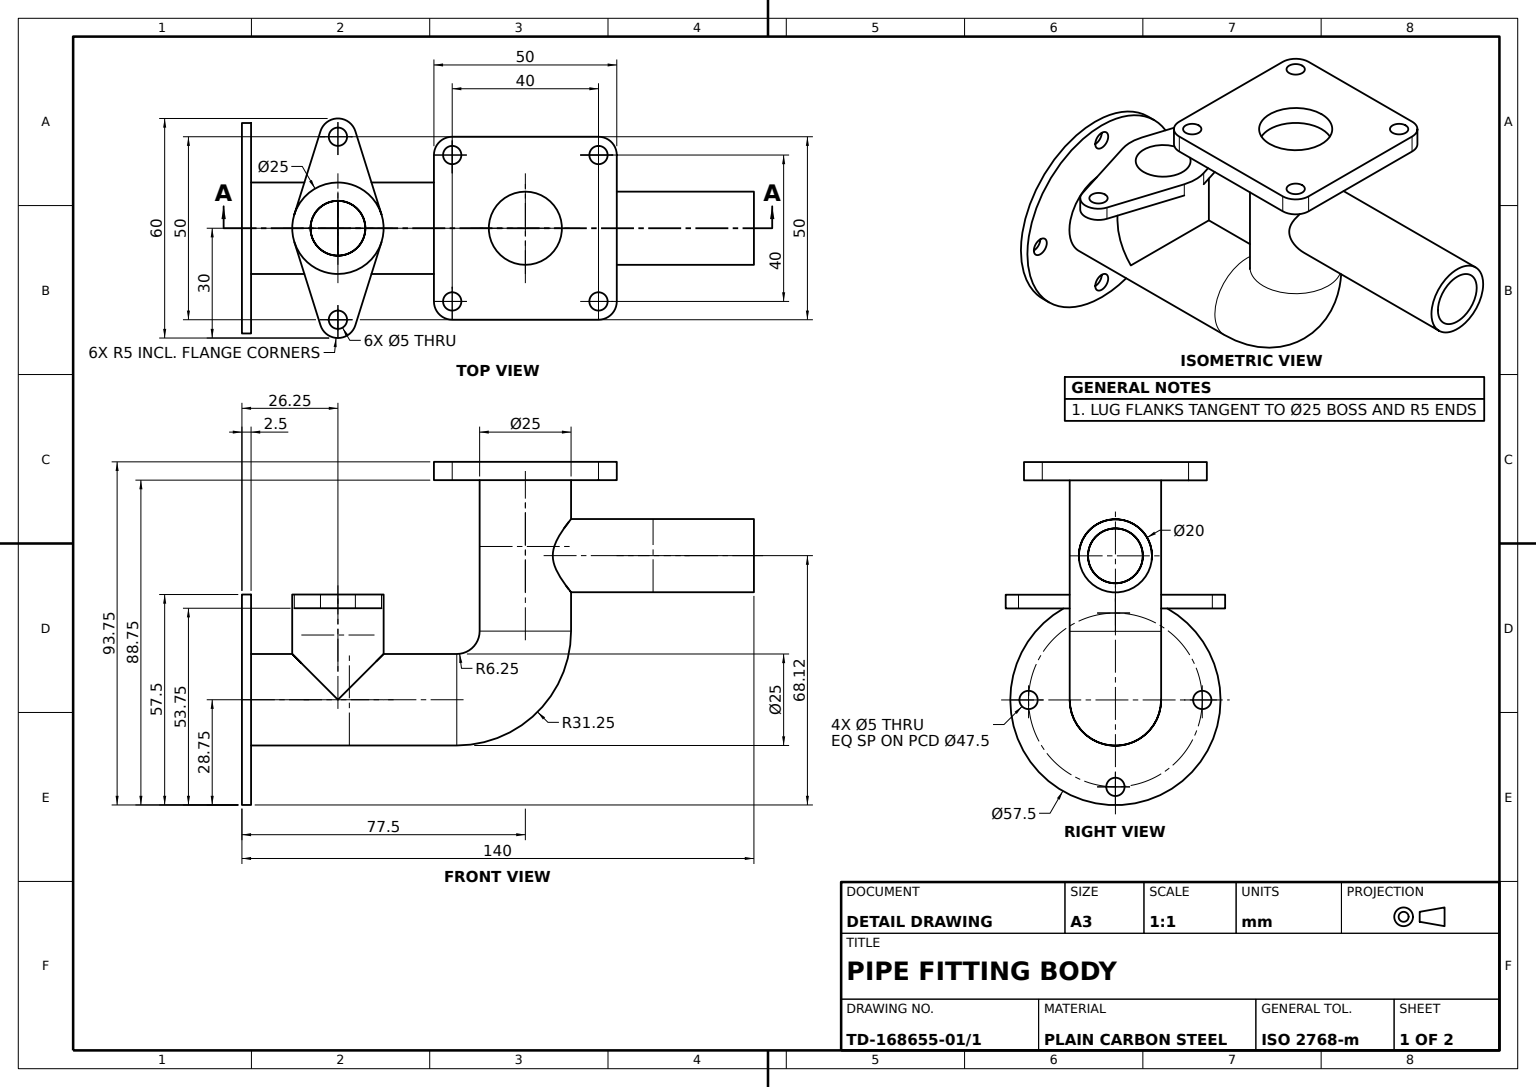
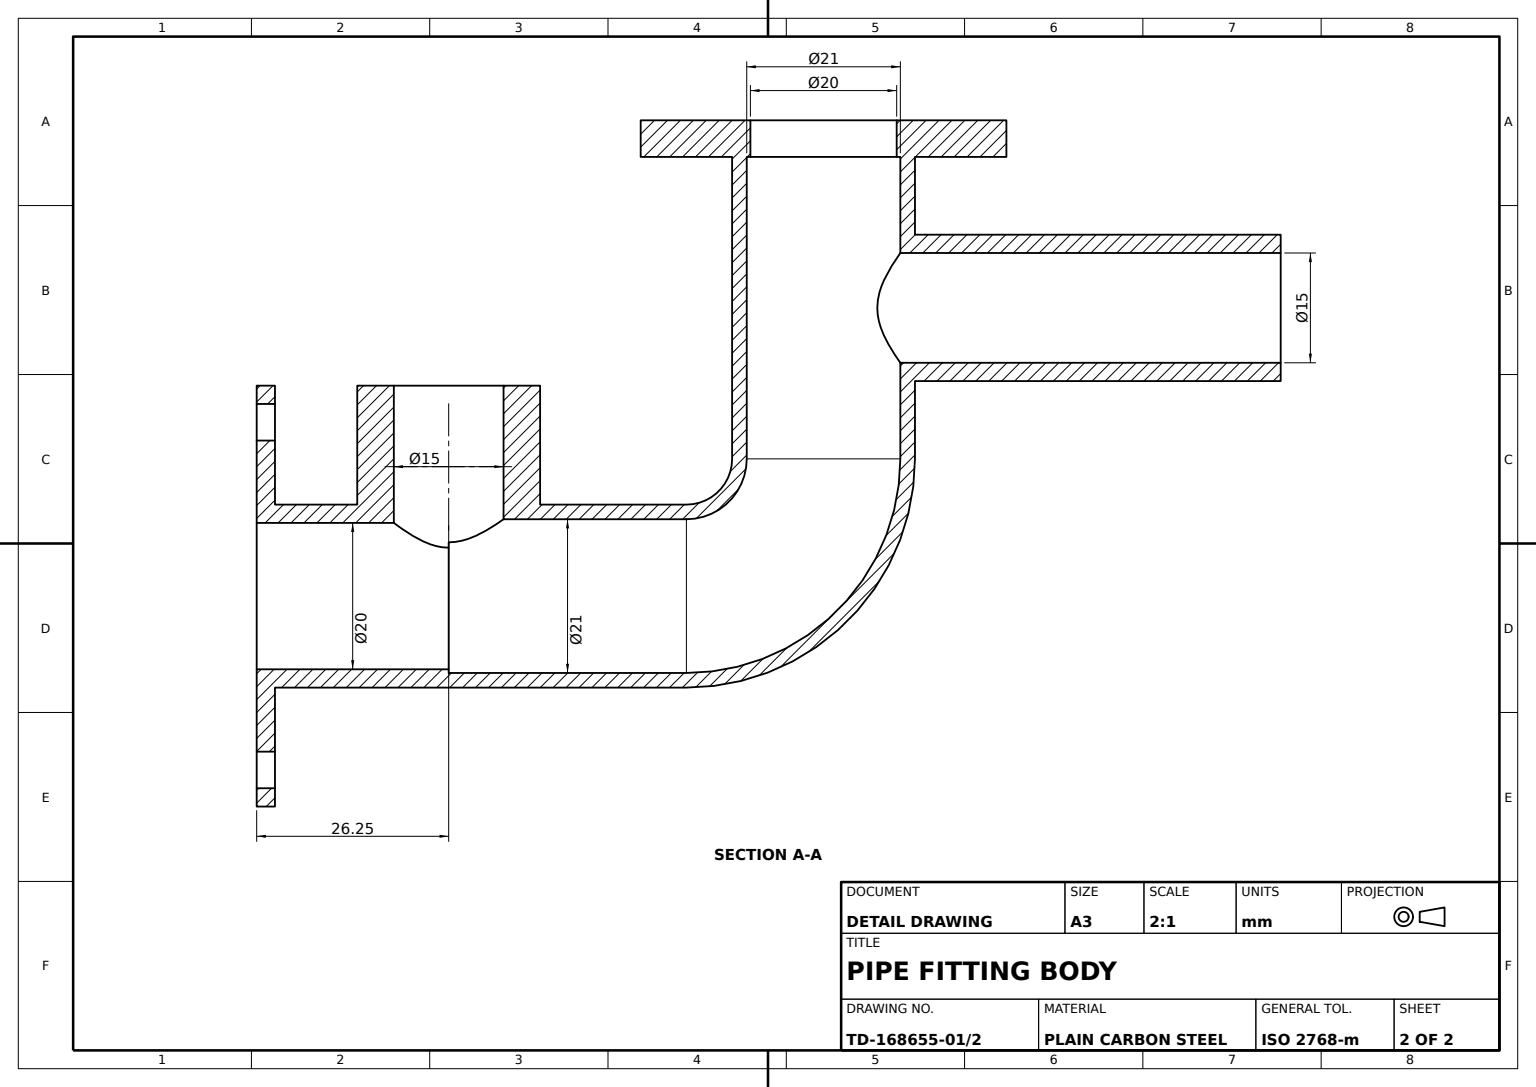
from build123d import *

# Parameters (mm, degrees)
ROUND_FLANGE_SKETCH_R         = 28.75
ROUND_FLANGE_57_5_DEPTH       = 2.5
INLET_PIPE_SKETCH_R           = 10
INLET_PIPE_20_DEPTH           = 23.75
FLANGE_A_NECK_REACH           = 71.44
FLANGE_A_NECK_END_RADIUS      = 10
FLANGE_A_NECK_SKETCH_R        = 10
FLANGE_A_HUB_SKETCH_R         = 12.5
FLANGE_A_HUB_25_DEPTH         = 3.75
FLANGE_A_LUG_1_SKETCH_R       = 5
FLANGE_A_LUG_1_DEPTH          = 3.75
FLANGE_A_LUG_2_SKETCH_R       = 5
FLANGE_A_LUG_2_DEPTH          = 3.75
FLANGE_A_WEB_25X10_DEPTH      = 3.75
FLANGE_A_TRIM_SKETCH_W        = 46.981578054
FLANGE_A_TRIM_SKETCH_H        = 84.080147296
FLANGE_A_TRIM_CUT_DEPTH       = 80
OUTLET_PIPE_SKETCH_R          = 12.5
OUTLET_PIPE_25_DEPTH          = 23.75
FLANGE_B_HUB_25_REACH         = 71.44
FLANGE_B_HUB_25_END_RADIUS    = 12.5
FLANGE_B_HUB_SKETCH_R         = 12.5
FLANGE_B_LUG_1_SKETCH_R       = 5
FLANGE_B_LUG_1_DEPTH          = 3.75
FLANGE_B_LUG_2_SKETCH_R       = 5
FLANGE_B_LUG_2_DEPTH          = 3.75
FLANGE_B_WEB_1_25X10_DEPTH    = 3.75
FLANGE_B_WEB_2_10X25_DEPTH    = 3.75
FLANGE_B_LUG_1_HOLE_SKETCH_R  = 2.5
FLANGE_B_LUG_1_HOLE_5_DEPTH   = 16.75
FLANGE_B_LUG_2_HOLE_SKETCH_R  = 2.5
FLANGE_B_LUG_2_HOLE_5_DEPTH   = 16.75
ELBOW_PIPE_SWEEP_PROFILE_R    = 12.5
ELBOW_PIPE_SWEEP_PROFILE_R_2  = 10.5
SQUARE_FLANGE_50X50_DEPTH     = 5
ROUND_FLANGE_BORE_SKETCH_R    = 10
ROUND_FLANGE_BORE_DEPTH       = 58
FLANGE_B_BORE_SKETCH_R        = 7.5
FLANGE_B_BORE_15_DEPTH        = 26
SQUARE_FLANGE_BORE_SKETCH_R   = 10
SQUARE_FLANGE_BORE_20_DEPTH   = 26
SQUARE_FLANGE_HOLE_1_SKETCH_R = 2.5
SQUARE_FLANGE_HOLE_1_5_DEPTH  = 26
SQUARE_FLANGE_HOLE_2_SKETCH_R = 2.5
SQUARE_FLANGE_HOLE_2_5_DEPTH  = 26
SQUARE_FLANGE_HOLE_3_SKETCH_R = 2.5
SQUARE_FLANGE_HOLE_3_5_DEPTH  = 26
SQUARE_FLANGE_HOLE_4_SKETCH_R = 2.5
SQUARE_FLANGE_HOLE_4_5_DEPTH  = 26
ROUND_FLANGE_HOLE_1_SKETCH_R  = 2.5
ROUND_FLANGE_HOLE_1_5_DEPTH   = 26
ROUND_FLANGE_HOLE_2_SKETCH_R  = 2.5
ROUND_FLANGE_HOLE_2_5_DEPTH   = 26
ROUND_FLANGE_HOLE_3_SKETCH_R  = 2.5
ROUND_FLANGE_HOLE_3_5_DEPTH   = 9
ROUND_FLANGE_HOLE_4_SKETCH_R  = 2.5
ROUND_FLANGE_HOLE_4_5_DEPTH   = 9
SIDE_PIPE_20_REACH            = 160.559
SIDE_PIPE_20_END_RADIUS       = 12.5
SIDE_PIPE_SKETCH_R            = 10
SIDE_PIPE_BORE_SKETCH_R       = 7.5
SIDE_PIPE_BORE_15_DEPTH       = 62


with BuildPart() as part:
    # Round Flange Sketch → Round Flange _57.5 (new body)
    with BuildSketch(Plane(origin=(0, 0, 0), x_dir=(0, 0, -1), z_dir=(1, 0, 0))):
        Circle(ROUND_FLANGE_SKETCH_R)
    extrude(amount=ROUND_FLANGE_57_5_DEPTH)

    # Inlet Pipe Sketch → Inlet Pipe _20 (add)
    with BuildSketch(Plane(origin=(2.5, 0, 0), x_dir=(0, 0, -1), z_dir=(1, 0, 0))):
        Circle(INLET_PIPE_SKETCH_R)
    extrude(amount=INLET_PIPE_20_DEPTH)

    # Flange A Neck: up to this cylinder (the profile starts outside it)
    flange_a_neck_end = Plane(origin=(26.25, 0, 0), z_dir=(-1, 0, 0)) * Cylinder(FLANGE_A_NECK_END_RADIUS, 163.88, mode=Mode.PRIVATE)
    # Flange A Neck Sketch → Flange A Neck (add, up to the surface)
    with BuildSketch(Plane(origin=(0, 28.75, 0), x_dir=(1, 0, 0), z_dir=(0, 1, 0)), mode=Mode.PRIVATE) as flange_a_neck_sk1:
        with Locations(Location((26.25, 0, 0), (0, 0, 270))):
            Circle(FLANGE_A_NECK_SKETCH_R)
    flange_a_neck_tool1 = extrude(flange_a_neck_sk1.sketch, amount=-FLANGE_A_NECK_REACH, mode=Mode.PRIVATE) - flange_a_neck_end
    add(flange_a_neck_tool1.solids().sort_by_distance((26.25, 28.75, 0))[0])

    # Flange A Hub Sketch → Flange A Hub _25 (add)
    with BuildSketch(Plane(origin=(0, 28.75, 0), x_dir=(1, 0, 0), z_dir=(0, 1, 0))):
        with Locations(Location((26.25, 0, 0), (0, 0, 270))):
            Circle(FLANGE_A_HUB_SKETCH_R)
    extrude(amount=-FLANGE_A_HUB_25_DEPTH)



with BuildPart() as body_2:
    # Flange A Lug 1 Sketch → Flange A Lug 1 (new body)
    with BuildSketch(Plane(origin=(0, 28.75, 0), x_dir=(1, 0, 0), z_dir=(0, 1, 0))):
        with Locations(Location((26.25, -25, 0), (0, 0, 270))):
            Circle(FLANGE_A_LUG_1_SKETCH_R)
    extrude(amount=-FLANGE_A_LUG_1_DEPTH)


with BuildPart() as body_3:
    # Flange A Lug 2 Sketch → Flange A Lug 2 (new body)
    with BuildSketch(Plane(origin=(0, 28.75, 0), x_dir=(1, 0, 0), z_dir=(0, 1, 0))):
        with Locations(Location((26.740993145, 25, 0), (0, 0, 270))):
            Circle(FLANGE_A_LUG_2_SKETCH_R)
    extrude(amount=-FLANGE_A_LUG_2_DEPTH)


with BuildPart() as part_1:
    add(part.part)

    add(body_2.part)  # Flange A Web 25x10 merges body 2
    # Flange A Web Sketch → Flange A Web 25x10 (add)
    with BuildSketch(Plane(origin=(0, 28.75, 0), x_dir=(1, 0, 0), z_dir=(0, 1, 0))):
        with BuildLine():
            ThreePointArc((38.174240018, -3.75), (26.25, -12.5), (14.325759982, -3.75))
            Line((14.325759982, -3.75), (21.480303993, -26.5))
            ThreePointArc((21.480303993, -26.5), (25.491211504, -20.057911371), (31.25, -25))
            ThreePointArc((31.25, -25), (31.192088629, -25.758788496), (31.019696007, -26.5))
            Line((31.019696007, -26.5), (38.174240018, -3.75))
        make_face()
    extrude(amount=-FLANGE_A_WEB_25X10_DEPTH)


with BuildPart() as flange_a_trim_cut_tool:
    # Flange A Trim Sketch → Flange A Trim Cut (new body)
    with BuildSketch(Plane(origin=(0, 28.75, 0), x_dir=(1, 0, 0), z_dir=(0, 1, 0))):
        with Locations((25.990789027, 3.010416982)):
            Rectangle(FLANGE_A_TRIM_SKETCH_W, FLANGE_A_TRIM_SKETCH_H)
    extrude(amount=-FLANGE_A_TRIM_CUT_DEPTH)


with BuildPart() as part_2:
    add(part_1.part)

    # Flange A Trim Cut: cut by flange_a_trim_cut_tool
    add(flange_a_trim_cut_tool.part, mode=Mode.SUBTRACT)

    # Outlet Pipe Sketch → Outlet Pipe _25 (add)
    with BuildSketch(Plane(origin=(2.5, 0, 0), x_dir=(0, 0, -1), z_dir=(1, 0, 0))):
        Circle(OUTLET_PIPE_SKETCH_R)
    extrude(amount=OUTLET_PIPE_25_DEPTH)

    # Flange B Hub _25: up to this cylinder (the profile starts outside it)
    flange_b_hub_25_end = Plane(origin=(26.25, 0, 0), z_dir=(-1, 0, 0)) * Cylinder(FLANGE_B_HUB_25_END_RADIUS, 168.88, mode=Mode.PRIVATE)
    # Flange B Hub Sketch → Flange B Hub _25 (add, up to the surface)
    with BuildSketch(Plane(origin=(0, 28.75, 0), x_dir=(1, 0, 0), z_dir=(0, 1, 0)), mode=Mode.PRIVATE) as flange_b_hub_25_sk1:
        with Locations(Location((26.25, 0, 0), (0, 0, 270))):
            Circle(FLANGE_B_HUB_SKETCH_R)
    flange_b_hub_25_tool1 = extrude(flange_b_hub_25_sk1.sketch, amount=-FLANGE_B_HUB_25_REACH, mode=Mode.PRIVATE) - flange_b_hub_25_end
    add(flange_b_hub_25_tool1.solids().sort_by_distance((26.25, 28.75, 0))[0])



with BuildPart() as body_3_1:
    add(body_3.part)

    # Flange A Trim Cut: cut by flange_a_trim_cut_tool
    add(flange_a_trim_cut_tool.part, mode=Mode.SUBTRACT)


with BuildPart() as body_2_2:
    # Flange B Lug 1 Sketch → Flange B Lug 1 (new body)
    with BuildSketch(Plane(origin=(0, 28.75, 0), x_dir=(1, 0, 0), z_dir=(0, 1, 0))):
        with Locations(Location((26.25, 25, 0), (0, 0, 270))):
            Circle(FLANGE_B_LUG_1_SKETCH_R)
    extrude(amount=-FLANGE_B_LUG_1_DEPTH)


with BuildPart() as body_3_2:
    # Flange B Lug 2 Sketch → Flange B Lug 2 (new body)
    with BuildSketch(Plane(origin=(0, 28.75, 0), x_dir=(1, 0, 0), z_dir=(0, 1, 0))):
        with Locations(Location((26.25, -25, 0), (0, 0, 270))):
            Circle(FLANGE_B_LUG_2_SKETCH_R)
    extrude(amount=-FLANGE_B_LUG_2_DEPTH)


with BuildPart() as part_3:
    add(part_2.part)

    add(body_2_2.part)  # Flange B Web 1 25x10 merges body 2 2
    # Flange B Web 1 Sketch → Flange B Web 1 25x10 (add)
    with BuildSketch(Plane(origin=(0, 28.75, 0), x_dir=(1, 0, 0), z_dir=(0, 1, 0))):
        with BuildLine():
            ThreePointArc((31.25, 25), (25.491211504, 20.057911371), (21.480303993, 26.5))
            Line((21.480303993, 26.5), (14.325759982, 3.75))
            ThreePointArc((14.325759982, 3.75), (26.25, 12.5), (38.174240018, 3.75))
            Line((38.174240018, 3.75), (31.019696007, 26.5))
            ThreePointArc((31.019696007, 26.5), (31.192088629, 25.758788496), (31.25, 25))
        make_face()
    extrude(amount=-FLANGE_B_WEB_1_25X10_DEPTH)


    add(body_3_2.part)  # Flange B Web 2 10x25 merges body 3 2
    # Flange B Web 2 Sketch → Flange B Web 2 10x25 (add)
    with BuildSketch(Plane(origin=(0, 28.75, 0), x_dir=(1, 0, 0), z_dir=(0, 1, 0))):
        with BuildLine():
            Line((14.325759982, -3.75), (21.480303993, -26.5))
            ThreePointArc((21.480303993, -26.5), (25.491211504, -20.057911371), (31.25, -25))
            ThreePointArc((31.25, -25), (31.192088629, -25.758788496), (31.019696007, -26.5))
            Line((31.019696007, -26.5), (38.174240018, -3.75))
            ThreePointArc((38.174240018, -3.75), (26.25, -12.5), (14.325759982, -3.75))
        make_face()
    extrude(amount=-FLANGE_B_WEB_2_10X25_DEPTH)

    # Flange B Lug 1 Hole Sketch → Flange B Lug 1 Hole _5 (cut)
    with BuildSketch(Plane(origin=(0, 28.75, 0), x_dir=(1, 0, 0), z_dir=(0, 1, 0))):
        with Locations(Location((26.25, 25, 0), (0, 0, 270))):
            Circle(FLANGE_B_LUG_1_HOLE_SKETCH_R)
    extrude(amount=-FLANGE_B_LUG_1_HOLE_5_DEPTH, mode=Mode.SUBTRACT)

    # Flange B Lug 2 Hole Sketch → Flange B Lug 2 Hole _5 (cut)
    with BuildSketch(Plane(origin=(0, 28.75, 0), x_dir=(1, 0, 0), z_dir=(0, 1, 0))):
        with Locations(Location((26.25, -25, 0), (0, 0, 270))):
            Circle(FLANGE_B_LUG_2_HOLE_SKETCH_R)
    extrude(amount=-FLANGE_B_LUG_2_HOLE_5_DEPTH, mode=Mode.SUBTRACT)

    # Elbow Pipe Sweep: sweep along a path in Elbow Path Sketch
    with BuildLine(Plane.XY) as elbow_pipe_sweep_path:
        Line((26.25, 0), (58.75, 0))
        ThreePointArc((58.75, 0), (72.008252147, 5.491747853), (77.5, 18.75))
        Line((77.5, 18.75), (77.5, 60))
    # Elbow Pipe Sweep profile (on start of the path) → Elbow Pipe Sweep (sweep)
    with BuildSketch(Plane(origin=(26.25, 0, 0), x_dir=(0, 0, 1), z_dir=(1, 0, 0))):
        Circle(ELBOW_PIPE_SWEEP_PROFILE_R)
        Circle(ELBOW_PIPE_SWEEP_PROFILE_R_2, mode=Mode.SUBTRACT)
    sweep(path=elbow_pipe_sweep_path.line)

    # Square Flange Sketch → Square Flange 50x50 (add)
    with BuildSketch(Plane(origin=(0, 60, 0), x_dir=(1, 0, 0), z_dir=(0, 1, 0))):
        with BuildLine():
            Line((57.5, 25), (97.5, 25))
            ThreePointArc((97.5, 25), (101.035533906, 23.535533906), (102.5, 20))
            Line((102.5, 20), (102.5, -20))
            ThreePointArc((102.5, -20), (101.035533906, -23.535533906), (97.5, -25))
            Line((97.5, -25), (57.5, -25))
            ThreePointArc((57.5, -25), (53.964466094, -23.535533906), (52.5, -20))
            Line((52.5, -20), (52.5, 20))
            ThreePointArc((52.5, 20), (53.964466094, 23.535533906), (57.5, 25))
        make_face()
    extrude(amount=SQUARE_FLANGE_50X50_DEPTH)

    # Round Flange Bore Sketch → Round Flange Bore (cut)
    with BuildSketch(Plane.ZY):
        Circle(ROUND_FLANGE_BORE_SKETCH_R)
    extrude(amount=-ROUND_FLANGE_BORE_DEPTH, mode=Mode.SUBTRACT)

    # Flange B Bore Sketch → Flange B Bore _15 (cut)
    with BuildSketch(Plane(origin=(0, 28.75, 0), x_dir=(1, 0, 0), z_dir=(0, 1, 0))):
        with Locations(Location((26.25, 0, 0), (0, 0, 270))):
            Circle(FLANGE_B_BORE_SKETCH_R)
    extrude(amount=-FLANGE_B_BORE_15_DEPTH, mode=Mode.SUBTRACT)

    # Square Flange Bore Sketch → Square Flange Bore _20 (cut)
    with BuildSketch(Plane(origin=(0, 65, 0), x_dir=(1, 0, 0), z_dir=(0, 1, 0))):
        with Locations(Location((77.5, 0, 0), (0, 0, 270))):
            Circle(SQUARE_FLANGE_BORE_SKETCH_R)
    extrude(amount=-SQUARE_FLANGE_BORE_20_DEPTH, mode=Mode.SUBTRACT)

    # Square Flange Hole 1 Sketch → Square Flange Hole 1 _5 (cut)
    with BuildSketch(Plane(origin=(0, 65, 0), x_dir=(1, 0, 0), z_dir=(0, 1, 0))):
        with Locations(Location((57.5, 20, 0), (0, 0, 270))):
            Circle(SQUARE_FLANGE_HOLE_1_SKETCH_R)
    extrude(amount=-SQUARE_FLANGE_HOLE_1_5_DEPTH, mode=Mode.SUBTRACT)

    # Square Flange Hole 2 Sketch → Square Flange Hole 2 _5 (cut)
    with BuildSketch(Plane(origin=(0, 65, 0), x_dir=(1, 0, 0), z_dir=(0, 1, 0))):
        with Locations(Location((57.5, -20, 0), (0, 0, 270))):
            Circle(SQUARE_FLANGE_HOLE_2_SKETCH_R)
    extrude(amount=-SQUARE_FLANGE_HOLE_2_5_DEPTH, mode=Mode.SUBTRACT)

    # Square Flange Hole 3 Sketch → Square Flange Hole 3 _5 (cut)
    with BuildSketch(Plane(origin=(0, 65, 0), x_dir=(1, 0, 0), z_dir=(0, 1, 0))):
        with Locations(Location((97.5, 20, 0), (0, 0, 270))):
            Circle(SQUARE_FLANGE_HOLE_3_SKETCH_R)
    extrude(amount=-SQUARE_FLANGE_HOLE_3_5_DEPTH, mode=Mode.SUBTRACT)

    # Square Flange Hole 4 Sketch → Square Flange Hole 4 _5 (cut)
    with BuildSketch(Plane(origin=(0, 65, 0), x_dir=(1, 0, 0), z_dir=(0, 1, 0))):
        with Locations(Location((97.5, -20, 0), (0, 0, 270))):
            Circle(SQUARE_FLANGE_HOLE_4_SKETCH_R)
    extrude(amount=-SQUARE_FLANGE_HOLE_4_5_DEPTH, mode=Mode.SUBTRACT)

    # Round Flange Hole 1 Sketch → Round Flange Hole 1 _5 (cut)
    with BuildSketch(Plane.ZY):
        with Locations((0, -23.75)):
            Circle(ROUND_FLANGE_HOLE_1_SKETCH_R)
    extrude(amount=-ROUND_FLANGE_HOLE_1_5_DEPTH, mode=Mode.SUBTRACT)

    # Round Flange Hole 2 Sketch → Round Flange Hole 2 _5 (cut)
    with BuildSketch(Plane.ZY):
        with Locations((-23.75, 0)):
            Circle(ROUND_FLANGE_HOLE_2_SKETCH_R)
    extrude(amount=-ROUND_FLANGE_HOLE_2_5_DEPTH, mode=Mode.SUBTRACT)

    # Round Flange Hole 3 Sketch → Round Flange Hole 3 _5 (cut)
    with BuildSketch(Plane.ZY):
        with Locations((0, 23.75)):
            Circle(ROUND_FLANGE_HOLE_3_SKETCH_R)
    extrude(amount=-ROUND_FLANGE_HOLE_3_5_DEPTH, mode=Mode.SUBTRACT)

    # Round Flange Hole 4 Sketch → Round Flange Hole 4 _5 (cut)
    with BuildSketch(Plane.ZY):
        with Locations((23.75, 0)):
            Circle(ROUND_FLANGE_HOLE_4_SKETCH_R)
    extrude(amount=-ROUND_FLANGE_HOLE_4_5_DEPTH, mode=Mode.SUBTRACT)

    # Side Pipe _20: up to this cylinder (the profile starts outside it)
    side_pipe_20_end = Plane(origin=(77.5, 39.375, 0), z_dir=(0, 1, 0)) * Cylinder(SIDE_PIPE_20_END_RADIUS, 347.118, mode=Mode.PRIVATE)
    # Side Pipe Sketch → Side Pipe _20 (add, up to the surface)
    with BuildSketch(Plane(origin=(140, 39.375, 0), x_dir=(0, 0, -1), z_dir=(1, 0, 0)), mode=Mode.PRIVATE) as side_pipe_20_sk1:
        Circle(SIDE_PIPE_SKETCH_R)
    side_pipe_20_tool1 = extrude(side_pipe_20_sk1.sketch, amount=-SIDE_PIPE_20_REACH, mode=Mode.PRIVATE) - side_pipe_20_end
    add(side_pipe_20_tool1.solids().sort_by_distance((140, 39.375, 0))[0])

    # Side Pipe Bore Sketch → Side Pipe Bore _15 (cut)
    with BuildSketch(Plane(origin=(140, 0, 0), x_dir=(0, 0, -1), z_dir=(1, 0, 0))):
        with Locations((0, 39.375)):
            Circle(SIDE_PIPE_BORE_SKETCH_R)
    extrude(amount=-SIDE_PIPE_BORE_15_DEPTH, mode=Mode.SUBTRACT)


solid = part_3.part
